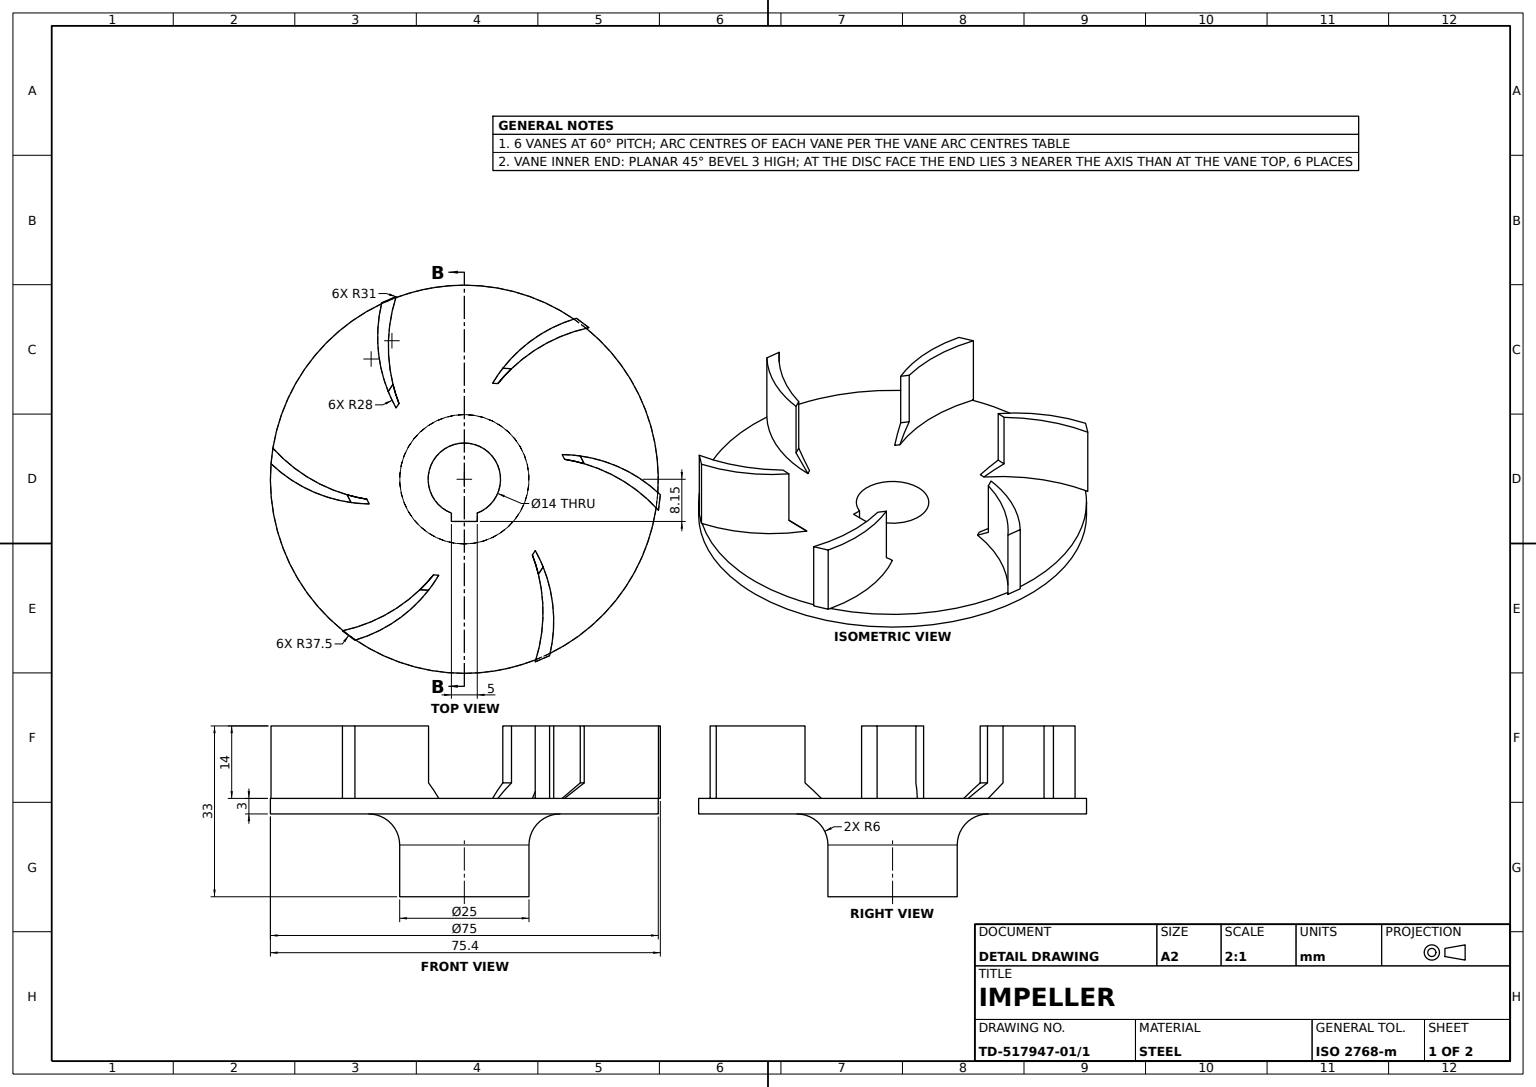
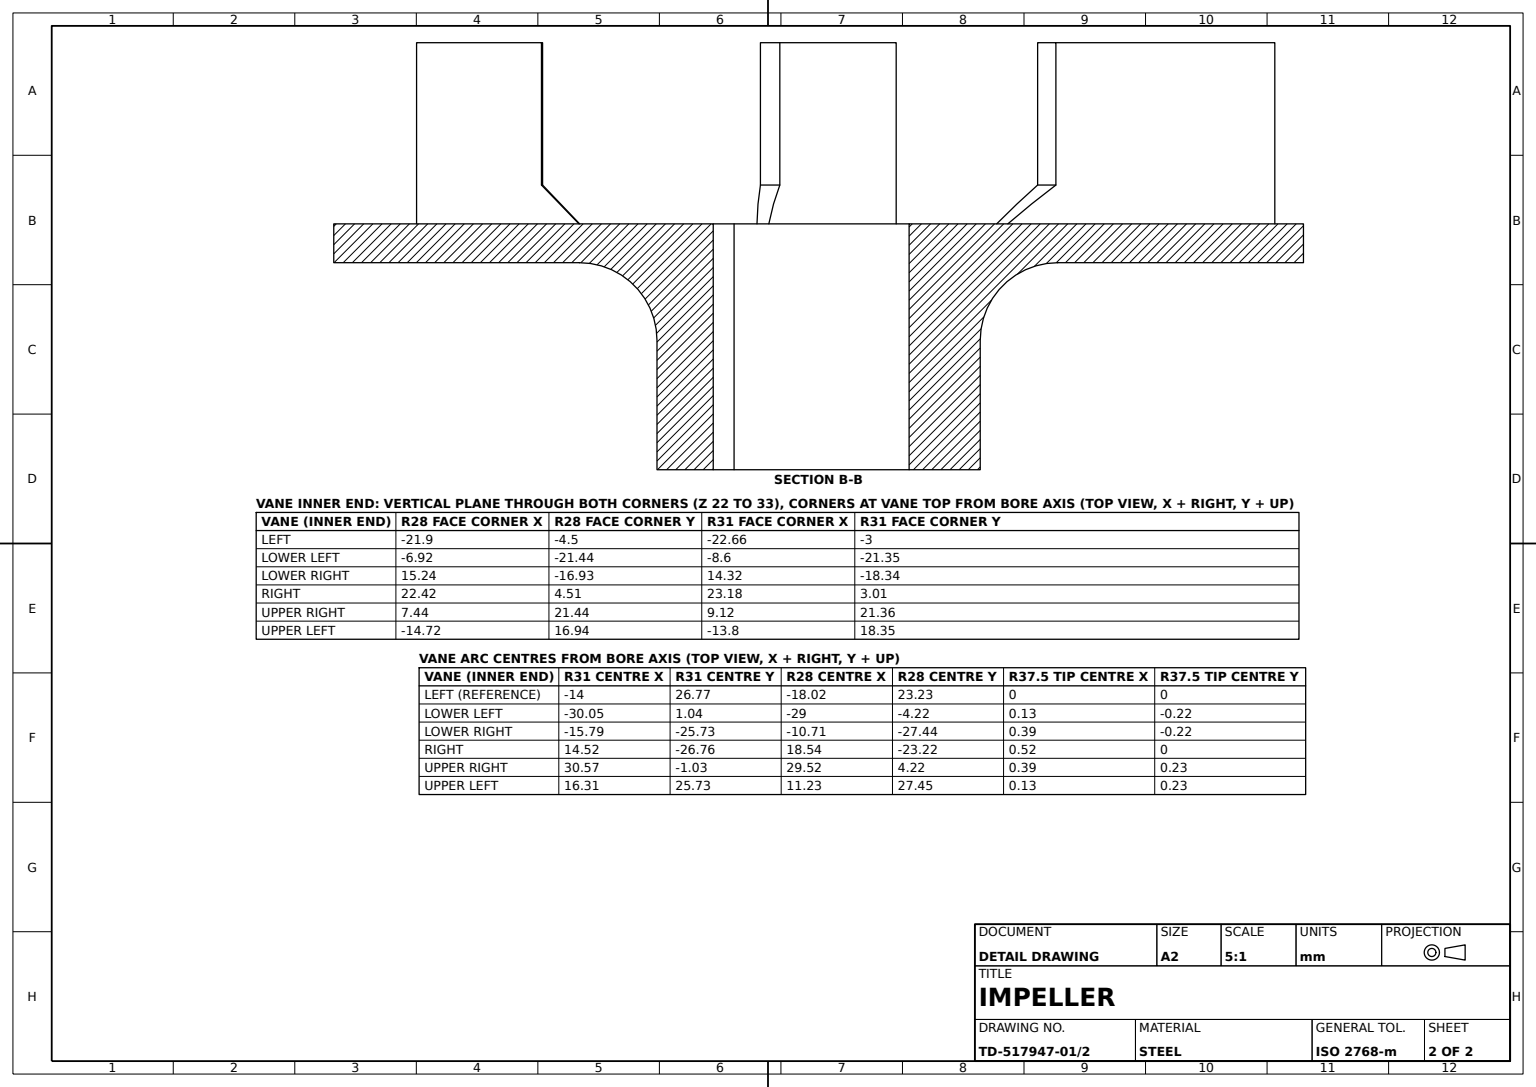
SolidWorks part; units mm, degrees
material "Plain Carbon Steel"
ref_plane "Front Plane" through (0, 0, 0) normal (0, 0, 1) x (1, 0, 0)
ref_plane "Top Plane" through (0, 0, 0) normal (0, 1, 0) x (1, 0, 0)
ref_plane "Right Plane" through (0, 0, 0) normal (1, 0, 0) x (0, 0, -1)
sketch "Base Disc Sketch" plane through (0, 0, 0) normal (0, 1, 0) x (1, 0, 0)
  circle A0 centre (0, 0) radius 37.5
  dimension "D1" = 75
extrude "Base Disc Ø75" add sketch "Base Disc Sketch" along normal blind 3
sketch "Vane Profile Sketch" plane through (0, 3, 0) normal (0, 1, 0) x (1, 0, 0)
  line L0 (0, 0) -> (-37.5, 0) construction
  line L1 (-22.6617, -3) -> (-21.8966, -4.5)
  circle A0 centre (0, 0) radius 37.5 construction
  arc A1 (-37.0169, 6) -> (-22.6617, -3) centre (-13.9993, 26.7651) ccw
  arc A2 (-37.3798, 3) -> (-21.8966, -4.5) centre (-18.0221, 23.2306) ccw
  arc A3 (-37.0169, 6) -> (-37.3798, 3) centre (0, 0) ccw
  dimension "D5" = 31
  dimension "D6" = 28
  dimension "D1" = 3
  dimension "D2" = 3
  dimension "D3" = 3
  dimension "D4" = 1.5
  dimension "D7" = 13.9993
  dimension "D8" = 18.0221
extrude "Vane" add sketch "Vane Profile Sketch" along normal blind 14
chamfer "Vane Chamfer 3mm" distance 3 angle 45 1 edges at (-22.2792, 3, 3.75)
pattern_circular "Vane Pattern 6x60°" count 6 every 60 about axis through (0.2597, 0, -0.0039) along (0, 1, 0) of "Vane", "Vane Chamfer 3mm"
sketch "Hub Sketch" plane through (0, 0, 0) normal (0, -1, 0) x (1, 0, 0)
  circle A0 centre (0, 0) radius 12.5
  dimension "D1" = 25
extrude "Hub Ø25" add sketch "Hub Sketch" along normal blind 16
sketch "Shaft Bore Sketch" plane through (0, -16, 0) normal (0, -1, 0) x (1, 0, 0)
  line L1 (-2.5, 8.15) -> (2.5, 8.15)
  line L2 (-2.5, 8.15) -> (-2.5, 6.5383)
  line L4 (2.5, 8.15) -> (2.5, 6.5383)
  arc A0 (-2.5, 6.5383) -> (2.5, 6.5383) centre (0, 0) ccw
  circle A1 centre (0, 0) radius 12.5 construction
  point P3 (0, 7)
  dimension "D1" = 14
  dimension "D3" = 8.15
  dimension "D2" = 5
extrude "Shaft Bore Ø14" cut sketch "Shaft Bore Sketch" against normal through all both and the other way through all
fillet "Hub Fillet R6" radius 6 1 edges at (0, 0, -12.5)
